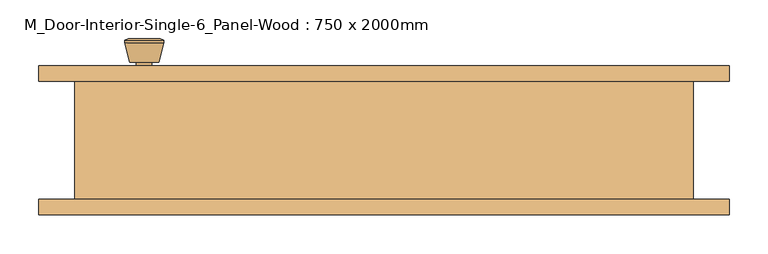
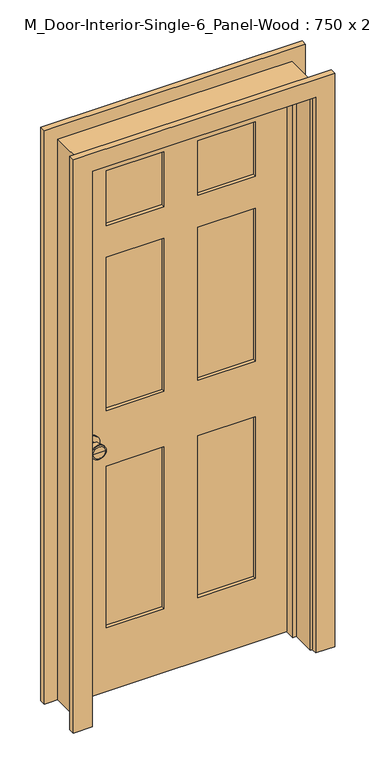
"""IFC4 building model written with IfcOpenShell, lengths in millimetres: door geometry, M_Door-Interior-Single-6_Panel-Wood : 750 x 2000mm."""

from ifc_helpers import new_model, si_unit, point, frame, frame_2d, origin, place, context, project, spatial, polyline, circle_curve, trimmed, segment, composite_curve, outline, extrude, faceted_brep, source, transform, mapped, element, save
from ifc_brep_helpers import plane_surface, cylinder_surface, revolved_surface, advanced_brep


def m_door_interior_single_6_panel_wood_750_x_2000mm_9b0189c3(model_context):
    return source(origin(), model_context, "Body", "SolidModel", [
        advanced_brep(
        [(-310.0, 32.025, 914.4), (-300.0, 32.025, 914.4), (-320.0, 32.025, 914.4), (-289.5241324, -16.975, 914.4), (-310.0, -16.975, 914.4), (-330.4758676, -16.975, 914.4), (-285.0, -15.1471319, 914.4), (-335.0, -15.1471319, 914.4), (-285.0, -11.6834537, 914.4), (-335.0, -11.6834537, 914.4), (-291.363764, 13.025, 914.4), (-328.636236, 13.025, 914.4), (-300.0, 13.025, 914.4), (-320.0, 13.025, 914.4)],
        [
            (0, 1),
            (1, 2, circle_curve(frame((-310.0, 32.025, 914.4), z_axis=(0.0, 1.0, 0.0), x_axis=(-1.0, 0.0, 0.0)), 10.0)),
            (2, 0),
            (2, 1, circle_curve(frame((-310.0, 32.025, 914.4), z_axis=(0.0, 1.0, 0.0), x_axis=(-1.0, 0.0, 0.0)), 10.0)),
            (3, 4),
            (4, 5),
            (5, 3, circle_curve(frame((-310.0, -16.975, 914.4), z_axis=(0.0, -1.0, 0.0), x_axis=(-1.0, 0.0, 0.0)), 20.4758676)),
            (3, 5, circle_curve(frame((-310.0, -16.975, 914.4), z_axis=(0.0, -1.0, 0.0), x_axis=(-1.0, 0.0, 0.0)), 20.4758676)),
            (6, 3),
            (5, 7),
            (7, 6, circle_curve(frame((-310.0, -15.1471319, 914.4), z_axis=(0.0, -1.0, 0.0), x_axis=(-1.0, 0.0, 0.0)), 25.0)),
            (6, 7, circle_curve(frame((-310.0, -15.1471319, 914.4), z_axis=(0.0, -1.0, 0.0), x_axis=(-1.0, 0.0, 0.0)), 25.0)),
            (8, 6),
            (7, 9),
            (9, 8, circle_curve(frame((-310.0, -11.6834537, 914.4), z_axis=(0.0, -1.0, 0.0), x_axis=(-1.0, 0.0, 0.0)), 25.0)),
            (8, 9, circle_curve(frame((-310.0, -11.6834537, 914.4), z_axis=(0.0, -1.0, 0.0), x_axis=(-1.0, 0.0, 0.0)), 25.0)),
            (10, 8),
            (9, 11),
            (11, 10, circle_curve(frame((-310.0, 13.025, 914.4), z_axis=(0.0, -1.0, 0.0), x_axis=(-1.0, 0.0, 0.0)), 18.636236)),
            (10, 11, circle_curve(frame((-310.0, 13.025, 914.4), z_axis=(0.0, -1.0, 0.0), x_axis=(-1.0, 0.0, 0.0)), 18.636236)),
            (12, 10),
            (11, 13),
            (13, 12, circle_curve(frame((-310.0, 13.025, 914.4), z_axis=(0.0, -1.0, 0.0), x_axis=(-1.0, 0.0, 0.0)), 10.0)),
            (12, 13, circle_curve(frame((-310.0, 13.025, 914.4), z_axis=(0.0, -1.0, 0.0), x_axis=(-1.0, 0.0, 0.0)), 10.0)),
            (1, 12),
            (13, 2),
        ],
        [
            plane_surface(frame((-310.0, 32.025, 914.4), z_axis=(0.0, 1.0, 0.0), x_axis=(-1.0, 0.0, 0.0))),
            plane_surface(frame((-310.0, -16.975, 914.4), z_axis=(0.0, -1.0, 0.0), x_axis=(-1.0, 0.0, 0.0))),
            revolved_surface(polyline([(-330.4758676, -16.975, 914.4), (-335.0, -15.1471319, 914.4)]), (-310.0, 32.025, 914.4), (0.0, 1.0, 0.0)),
            cylinder_surface(frame((-310.0, 32.025, 914.4), z_axis=(0.0, 1.0, 0.0), x_axis=(-1.0, 0.0, 0.0)), 25.0),
            revolved_surface(polyline([(-335.0, -11.6834537, 914.4), (-328.636236, 13.025, 914.4)]), (-310.0, 32.025, 914.4), (0.0, 1.0, 0.0)),
            plane_surface(frame((-310.0, 13.025, 914.4), z_axis=(0.0, 1.0, 0.0), x_axis=(-1.0, 0.0, 0.0))),
            cylinder_surface(frame((-310.0, 32.025, 914.4), z_axis=(0.0, 1.0, 0.0), x_axis=(-1.0, 0.0, 0.0)), 10.0),
        ],
        [
            (0, [[1, 2, 3]]),
            (0, [[-3, 4, -1]]),
            (1, [[5, 6, 7]]),
            (1, [[-6, -5, 8]]),
            (2, [[9, -7, 10, 11]]),
            (2, [[-10, -8, -9, 12]]),
            (3, [[13, -11, 14, 15]]),
            (3, [[-14, -12, -13, 16]]),
            (4, [[17, -15, 18, 19]]),
            (4, [[-18, -16, -17, 20]]),
            (5, [[21, -19, 22, 23]]),
            (5, [[-22, -20, -21, 24]]),
            (6, [[25, -23, 26, -2]]),
            (6, [[-26, -24, -25, -4]]),
        ],
    ),
        extrude(outline(composite_curve([segment(trimmed(circle_curve(frame_2d((914.4, -310.0)), 30.0), [point((914.4, -340.0))], [point((914.4, -280.0))], False, "CARTESIAN"), True, "CONTINUOUS"), segment(trimmed(circle_curve(frame_2d((914.4, -310.0)), 30.0), [point((914.4, -280.0))], [point((914.4, -340.0))], False, "CARTESIAN"), True, "CONTINUOUS")], self_intersect=False)), frame((0.0, 32.025, 0.0), z_axis=(0.0, 1.0, 0.0), x_axis=(0.0, 0.0, 1.0)), (0.0, 0.0, 1.0), 6.0),
        advanced_brep(
        [(-310.0, 79.025, 914.4), (-320.0, 79.025, 914.4), (-300.0, 79.025, 914.4), (-289.5241324, 128.025, 914.4), (-330.4758676, 128.025, 914.4), (-310.0, 128.025, 914.4), (-285.0, 126.1971319, 914.4), (-335.0, 126.1971319, 914.4), (-285.0, 122.7334537, 914.4), (-335.0, 122.7334537, 914.4), (-291.363764, 98.025, 914.4), (-328.636236, 98.025, 914.4), (-300.0, 98.025, 914.4), (-320.0, 98.025, 914.4)],
        [
            (0, 1),
            (1, 2, circle_curve(frame((-310.0, 79.025, 914.4), z_axis=(0.0, -1.0, 0.0), x_axis=(-1.0, 0.0, 0.0)), 10.0)),
            (2, 0),
            (2, 1, circle_curve(frame((-310.0, 79.025, 914.4), z_axis=(0.0, -1.0, 0.0), x_axis=(-1.0, 0.0, 0.0)), 10.0)),
            (3, 4, circle_curve(frame((-310.0, 128.025, 914.4), z_axis=(0.0, 1.0, 0.0), x_axis=(-1.0, 0.0, 0.0)), 20.4758676)),
            (4, 5),
            (5, 3),
            (4, 3, circle_curve(frame((-310.0, 128.025, 914.4), z_axis=(0.0, 1.0, 0.0), x_axis=(-1.0, 0.0, 0.0)), 20.4758676)),
            (6, 7, circle_curve(frame((-310.0, 126.1971319, 914.4), z_axis=(0.0, 1.0, 0.0), x_axis=(-1.0, 0.0, 0.0)), 25.0)),
            (7, 4),
            (3, 6),
            (7, 6, circle_curve(frame((-310.0, 126.1971319, 914.4), z_axis=(0.0, 1.0, 0.0), x_axis=(-1.0, 0.0, 0.0)), 25.0)),
            (8, 9, circle_curve(frame((-310.0, 122.7334537, 914.4), z_axis=(0.0, 1.0, 0.0), x_axis=(-1.0, 0.0, 0.0)), 25.0)),
            (9, 7),
            (6, 8),
            (9, 8, circle_curve(frame((-310.0, 122.7334537, 914.4), z_axis=(0.0, 1.0, 0.0), x_axis=(-1.0, 0.0, 0.0)), 25.0)),
            (10, 11, circle_curve(frame((-310.0, 98.025, 914.4), z_axis=(0.0, 1.0, 0.0), x_axis=(-1.0, 0.0, 0.0)), 18.636236)),
            (11, 9),
            (8, 10),
            (11, 10, circle_curve(frame((-310.0, 98.025, 914.4), z_axis=(0.0, 1.0, 0.0), x_axis=(-1.0, 0.0, 0.0)), 18.636236)),
            (12, 13, circle_curve(frame((-310.0, 98.025, 914.4), z_axis=(0.0, 1.0, 0.0), x_axis=(-1.0, 0.0, 0.0)), 10.0)),
            (13, 11),
            (10, 12),
            (13, 12, circle_curve(frame((-310.0, 98.025, 914.4), z_axis=(0.0, 1.0, 0.0), x_axis=(-1.0, 0.0, 0.0)), 10.0)),
            (1, 13),
            (12, 2),
        ],
        [
            plane_surface(frame((-310.0, 79.025, 914.4), z_axis=(0.0, -1.0, 0.0), x_axis=(-1.0, 0.0, 0.0))),
            plane_surface(frame((-310.0, 128.025, 914.4), z_axis=(0.0, 1.0, 0.0), x_axis=(-1.0, 0.0, 0.0))),
            revolved_surface(polyline([(-330.4758676, 128.025, 914.4), (-335.0, 126.1971319, 914.4)]), (-310.0, 79.025, 914.4), (0.0, -1.0, 0.0)),
            cylinder_surface(frame((-310.0, 79.025, 914.4), z_axis=(0.0, -1.0, 0.0), x_axis=(-1.0, 0.0, 0.0)), 25.0),
            revolved_surface(polyline([(-335.0, 122.7334537, 914.4), (-328.636236, 98.025, 914.4)]), (-310.0, 79.025, 914.4), (0.0, -1.0, 0.0)),
            plane_surface(frame((-310.0, 98.025, 914.4), z_axis=(0.0, -1.0, 0.0), x_axis=(-1.0, 0.0, 0.0))),
            cylinder_surface(frame((-310.0, 79.025, 914.4), z_axis=(0.0, -1.0, 0.0), x_axis=(-1.0, 0.0, 0.0)), 10.0),
        ],
        [
            (0, [[1, 2, 3]]),
            (0, [[-3, 4, -1]]),
            (1, [[5, 6, 7]]),
            (1, [[8, -7, -6]]),
            (2, [[9, 10, -5, 11]]),
            (2, [[12, -11, -8, -10]]),
            (3, [[13, 14, -9, 15]]),
            (3, [[16, -15, -12, -14]]),
            (4, [[17, 18, -13, 19]]),
            (4, [[20, -19, -16, -18]]),
            (5, [[21, 22, -17, 23]]),
            (5, [[24, -23, -20, -22]]),
            (6, [[-2, 25, -21, 26]]),
            (6, [[-4, -26, -24, -25]]),
        ],
    ),
        extrude(outline(composite_curve([segment(trimmed(circle_curve(frame_2d((914.4, -310.0)), 30.0), [point((914.4, -340.0))], [point((914.4, -280.0))], False, "CARTESIAN"), True, "CONTINUOUS"), segment(trimmed(circle_curve(frame_2d((914.4, -310.0)), 30.0), [point((914.4, -280.0))], [point((914.4, -340.0))], False, "CARTESIAN"), True, "CONTINUOUS")], self_intersect=False)), frame((0.0, 73.025, 0.0), z_axis=(0.0, 1.0, 0.0), x_axis=(0.0, 0.0, 1.0)), (0.0, 0.0, 1.0), 6.0),
        faceted_brep([(400.0, 73.025, 0.0), (400.0, -79.375, 0.0), (375.0, -79.375, 0.0), (375.0, 3.1, 0.0), (362.3, 3.1, 0.0), (362.3, 38.025, 0.0), (375.0, 38.025, 0.0), (375.0, 73.025, 0.0), (400.0, 73.025, 2025.0), (400.0, -79.375, 2025.0), (-400.0, -79.375, 2025.0), (-400.0, -79.375, 0.0), (-375.0, -79.375, 0.0), (-375.0, -79.375, 2000.0), (375.0, -79.375, 2000.0), (375.0, 3.1, 2000.0), (-375.0, 3.1, 2000.0), (-375.0, 3.1, 0.0), (-362.3, 3.1, 0.0), (-362.3, 3.1, 1987.3), (362.3, 3.1, 1987.3), (362.3, 38.025, 1987.3), (-362.3, 38.025, 1987.3), (-362.3, 38.025, 0.0), (-375.0, 38.025, 0.0), (-375.0, 38.025, 2000.0), (375.0, 38.025, 2000.0), (375.0, 73.025, 2000.0), (-375.0, 73.025, 2000.0), (-375.0, 73.025, 0.0), (-400.0, 73.025, 0.0), (-400.0, 73.025, 2025.0)], [[[0, 1, 2, 3, 4, 5, 6, 7]], [[1, 0, 8, 9]], [[2, 1, 9, 10, 11, 12, 13, 14]], [[3, 2, 14, 15]], [[4, 3, 15, 16, 17, 18, 19, 20]], [[5, 4, 20, 21]], [[6, 5, 21, 22, 23, 24, 25, 26]], [[7, 6, 26, 27]], [[0, 7, 27, 28, 29, 30, 31, 8]], [[9, 8, 31, 10]], [[15, 14, 13, 16]], [[21, 20, 19, 22]], [[27, 26, 25, 28]], [[30, 29, 24, 23, 18, 17, 12, 11]], [[10, 31, 30, 11]], [[16, 13, 12, 17]], [[22, 19, 18, 23]], [[28, 25, 24, 29]]]),
        extrude(outline(polyline([(2000.0, -375.0), (0.0, -375.0), (0.0, 375.0), (2000.0, 375.0), (2000.0, -375.0)]), holes=[polyline([(1880.0, 57.5), (1880.0, 255.0), (1682.5, 255.0), (1682.5, 57.5), (1880.0, 57.5)]), polyline([(1567.5, 255.0), (1014.4, 255.0), (1014.4, 57.5), (1567.5, 57.5), (1567.5, 255.0)]), polyline([(1014.4, -57.5), (1014.4, -255.0), (1567.5, -255.0), (1567.5, -57.5), (1014.4, -57.5)]), polyline([(1682.5, -255.0), (1880.0, -255.0), (1880.0, -57.5), (1682.5, -57.5), (1682.5, -255.0)]), polyline([(814.4, 57.5), (814.4, 255.0), (230.0, 255.0), (230.0, 57.5), (814.4, 57.5)]), polyline([(230.0, -57.5), (230.0, -255.0), (814.4, -255.0), (814.4, -57.5), (230.0, -57.5)])]), frame((0.0, 38.025, 0.0), z_axis=(0.0, 1.0, 0.0), x_axis=(0.0, 0.0, 1.0)), (0.0, 0.0, 1.0), 35.0),
        extrude(outline(polyline([(255.0, 49.6916667), (57.5, 49.6916667), (57.5, 61.3583333), (255.0, 61.3583333), (255.0, 49.6916667)])), frame((0.0, 0.0, 1682.5), z_axis=(0.0, 0.0, 1.0), x_axis=(1.0, 0.0, 0.0)), (0.0, 0.0, 1.0), 197.5),
        extrude(outline(polyline([(255.0, 49.6916667), (57.5, 49.6916667), (57.5, 61.3583333), (255.0, 61.3583333), (255.0, 49.6916667)])), frame((0.0, 0.0, 1014.4), z_axis=(0.0, 0.0, 1.0), x_axis=(1.0, 0.0, 0.0)), (0.0, 0.0, 1.0), 553.1),
        extrude(outline(polyline([(-57.5, 49.6916667), (-255.0, 49.6916667), (-255.0, 61.3583333), (-57.5, 61.3583333), (-57.5, 49.6916667)])), frame((0.0, 0.0, 1014.4), z_axis=(0.0, 0.0, 1.0), x_axis=(1.0, 0.0, 0.0)), (0.0, 0.0, 1.0), 553.1),
        extrude(outline(polyline([(-57.5, 49.6916667), (-255.0, 49.6916667), (-255.0, 61.3583333), (-57.5, 61.3583333), (-57.5, 49.6916667)])), frame((0.0, 0.0, 1682.5), z_axis=(0.0, 0.0, 1.0), x_axis=(1.0, 0.0, 0.0)), (0.0, 0.0, 1.0), 197.5),
        extrude(outline(polyline([(255.0, 49.6916667), (57.5, 49.6916667), (57.5, 61.3583333), (255.0, 61.3583333), (255.0, 49.6916667)])), frame((0.0, 0.0, 230.0), z_axis=(0.0, 0.0, 1.0), x_axis=(1.0, 0.0, 0.0)), (0.0, 0.0, 1.0), 584.4),
        extrude(outline(polyline([(-57.5, 49.6916667), (-255.0, 49.6916667), (-255.0, 61.3583333), (-57.5, 61.3583333), (-57.5, 49.6916667)])), frame((0.0, 0.0, 230.0), z_axis=(0.0, 0.0, 1.0), x_axis=(1.0, 0.0, 0.0)), (0.0, 0.0, 1.0), 584.4),
        extrude(outline(polyline([(0.0, 381.35), (0.0, 446.35), (2071.35, 446.35), (2071.35, -446.35), (0.0, -446.35), (0.0, -381.35), (2006.35, -381.35), (2006.35, 381.35), (0.0, 381.35)])), frame((0.0, 73.025, 0.0), z_axis=(0.0, 1.0, 0.0), x_axis=(0.0, 0.0, 1.0)), (0.0, 0.0, 1.0), 20.0),
        extrude(outline(polyline([(0.0, 381.35), (0.0, 446.35), (2071.35, 446.35), (2071.35, -446.35), (0.0, -446.35), (0.0, -381.35), (2006.35, -381.35), (2006.35, 381.35), (0.0, 381.35)])), frame((0.0, -99.375, 0.0), z_axis=(0.0, 1.0, 0.0), x_axis=(0.0, 0.0, 1.0)), (0.0, 0.0, 1.0), 20.0),
    ])


if __name__ == "__main__":
    model = new_model("IFC4")
    model_context = context("Model", 3, world=origin())
    ifc_project = project(units=[si_unit("LENGTHUNIT", "METRE", prefix="MILLI")], contexts=[model_context])
    site = spatial("IfcSite", under=ifc_project)
    building = spatial("IfcBuilding", under=site)
    placement = place(None, origin())
    m_door_interior_single_6_panel_wood_750_x_2000mm_shape = m_door_interior_single_6_panel_wood_750_x_2000mm_9b0189c3(model_context)
    element("IfcDoor", 1, ObjectType="M_Door-Interior-Single-6_Panel-Wood : 750 x 2000mm", at=placement, inside=building, context=model_context, shape_type="MappedRepresentation", body=[
        mapped(m_door_interior_single_6_panel_wood_750_x_2000mm_shape, transform((0.0, 0.0, 0.0), x_axis=(1.0, 0.0, 0.0), y_axis=(0.0, 1.0, 0.0), z_axis=(0.0, 0.0, 1.0))),
    ])
    save(model, "model.ifc")

# Revit data of these elements
# Type "M_Door-Interior-Single-6_Panel-Wood : 750 x 2000mm"
#   Type Mark = "10"
#   Assembly Code = "C1020300"
#   Analytic Construction = "Wooden"
#   Top Rail = 0' - 4.72441"
#   Top Panel = 0' - 7.77559"
#   Thickness = 0' - 1.37795"
#   Thermal Resistance (R) = 2.5876 (h·ft²·°F)/BTU
#   Swing Angle [instance default] = 90.00°
#   Stiles = 0' - 4.72441"
#   Rough Width = 2' - 7.49606"
#   Rough Height = 6' - 7.72441"
#   Mullion = 0' - 4.52756"
#   Lock Rail = 0' - 7.87402"
#   Intermediate Rail = 0' - 4.52756"
#   Height = 6' - 6.74016"
#   Width = 2' - 5.52756"
#   Heat Transfer Coefficient (U) = 0.3865 BTU/(h·ft²·°F)
#   Bottom Rail = 0' - 9.05512"
#   Trim Material = Cherry
#   Panel Material = Cherry
#   Frame Material = Cherry
#   Door Handle Material = Aluminum
#   Visual Light Transmittance = 0
#   Solar Heat Gain Coefficient = 0
#   Wall Closure = (empty or 0)
#   Function = (empty or 0)
# Element 1 (IfcDoor, "M_Door-Interior-Single-6_Panel-Wood : 750 x 2000mm")
#   Materials on its faces: "Cherry", "Aluminum"
# Materials
#   "Cherry": class "Wood", colour RGB 226 177 128, transparency 0, Description = "Prunus Serotina", Cost = 0
#   "Aluminum": class "Metal", colour RGB 247 247 247, transparency 0, Description = "Aluminum 6061", Cost = 0
